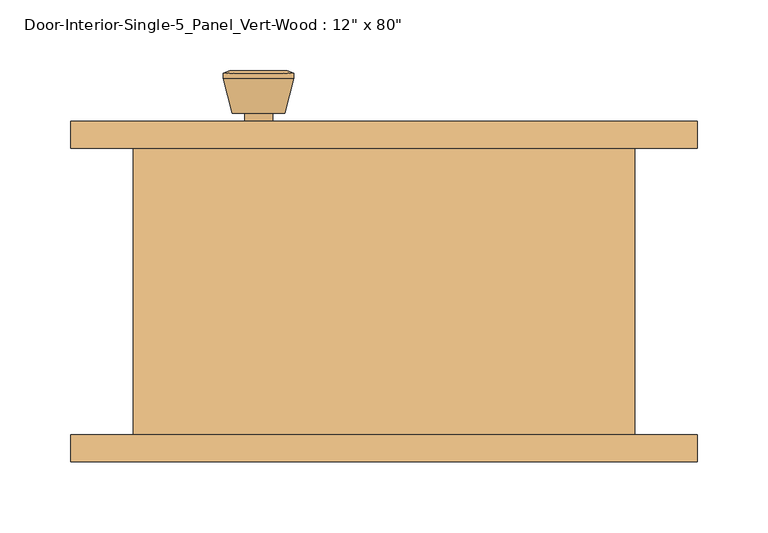
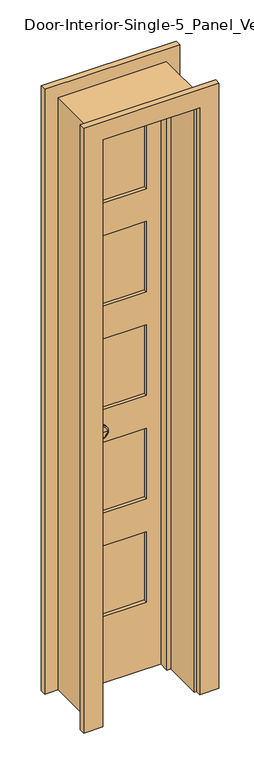
"""IFC4 building model written with IfcOpenShell, lengths in millimetres: door geometry."""

from ifc_helpers import new_model, si_unit, point, frame, frame_2d, origin, place, context, project, spatial, polyline, circle_curve, trimmed, segment, composite_curve, outline, extrude, faceted_brep, source, transform, mapped, element, save
from ifc_brep_helpers import plane_surface, cylinder_surface, revolved_surface, advanced_brep


def door_5a382651(model_context):
    return source(origin(), model_context, "Body", "SolidModel", [
        advanced_brep(
        [(-88.9, 57.5, 914.4), (-78.9, 57.5, 914.4), (-98.9, 57.5, 914.4), (-68.4241324, 8.5, 914.4), (-88.9, 8.5, 914.4), (-109.3758676, 8.5, 914.4), (-63.9, 10.3278681, 914.4), (-113.9, 10.3278681, 914.4), (-63.9, 13.7915463, 914.4), (-113.9, 13.7915463, 914.4), (-70.263764, 38.5, 914.4), (-107.536236, 38.5, 914.4), (-78.9, 38.5, 914.4), (-98.9, 38.5, 914.4)],
        [
            (0, 1),
            (1, 2, circle_curve(frame((-88.9, 57.5, 914.4), z_axis=(0.0, 1.0, 0.0), x_axis=(-1.0, 0.0, 0.0)), 10.0)),
            (2, 0),
            (2, 1, circle_curve(frame((-88.9, 57.5, 914.4), z_axis=(0.0, 1.0, 0.0), x_axis=(-1.0, 0.0, 0.0)), 10.0)),
            (3, 4),
            (4, 5),
            (5, 3, circle_curve(frame((-88.9, 8.5, 914.4), z_axis=(0.0, -1.0, 0.0), x_axis=(-1.0, 0.0, 0.0)), 20.4758676)),
            (3, 5, circle_curve(frame((-88.9, 8.5, 914.4), z_axis=(0.0, -1.0, 0.0), x_axis=(-1.0, 0.0, 0.0)), 20.4758676)),
            (6, 3),
            (5, 7),
            (7, 6, circle_curve(frame((-88.9, 10.3278681, 914.4), z_axis=(0.0, -1.0, 0.0), x_axis=(-1.0, 0.0, 0.0)), 25.0)),
            (6, 7, circle_curve(frame((-88.9, 10.3278681, 914.4), z_axis=(0.0, -1.0, 0.0), x_axis=(-1.0, 0.0, 0.0)), 25.0)),
            (8, 6),
            (7, 9),
            (9, 8, circle_curve(frame((-88.9, 13.7915463, 914.4), z_axis=(0.0, -1.0, 0.0), x_axis=(-1.0, 0.0, 0.0)), 25.0)),
            (8, 9, circle_curve(frame((-88.9, 13.7915463, 914.4), z_axis=(0.0, -1.0, 0.0), x_axis=(-1.0, 0.0, 0.0)), 25.0)),
            (10, 8),
            (9, 11),
            (11, 10, circle_curve(frame((-88.9, 38.5, 914.4), z_axis=(0.0, -1.0, 0.0), x_axis=(-1.0, 0.0, 0.0)), 18.636236)),
            (10, 11, circle_curve(frame((-88.9, 38.5, 914.4), z_axis=(0.0, -1.0, 0.0), x_axis=(-1.0, 0.0, 0.0)), 18.636236)),
            (12, 10),
            (11, 13),
            (13, 12, circle_curve(frame((-88.9, 38.5, 914.4), z_axis=(0.0, -1.0, 0.0), x_axis=(-1.0, 0.0, 0.0)), 10.0)),
            (12, 13, circle_curve(frame((-88.9, 38.5, 914.4), z_axis=(0.0, -1.0, 0.0), x_axis=(-1.0, 0.0, 0.0)), 10.0)),
            (1, 12),
            (13, 2),
        ],
        [
            plane_surface(frame((-88.9, 57.5, 914.4), z_axis=(0.0, 1.0, 0.0), x_axis=(-1.0, 0.0, 0.0))),
            plane_surface(frame((-88.9, 8.5, 914.4), z_axis=(0.0, -1.0, 0.0), x_axis=(-1.0, 0.0, 0.0))),
            revolved_surface(polyline([(-109.3758676, 8.5, 914.4), (-113.9, 10.3278681, 914.4)]), (-88.9, 57.5, 914.4), (0.0, 1.0, 0.0)),
            cylinder_surface(frame((-88.9, 57.5, 914.4), z_axis=(0.0, 1.0, 0.0), x_axis=(-1.0, 0.0, 0.0)), 25.0),
            revolved_surface(polyline([(-113.9, 13.7915463, 914.4), (-107.536236, 38.5, 914.4)]), (-88.9, 57.5, 914.4), (0.0, 1.0, 0.0)),
            plane_surface(frame((-88.9, 38.5, 914.4), z_axis=(0.0, 1.0, 0.0), x_axis=(-1.0, 0.0, 0.0))),
            cylinder_surface(frame((-88.9, 57.5, 914.4), z_axis=(0.0, 1.0, 0.0), x_axis=(-1.0, 0.0, 0.0)), 10.0),
        ],
        [
            (0, [[1, 2, 3]]),
            (0, [[-3, 4, -1]]),
            (1, [[5, 6, 7]]),
            (1, [[-6, -5, 8]]),
            (2, [[9, -7, 10, 11]]),
            (2, [[-10, -8, -9, 12]]),
            (3, [[13, -11, 14, 15]]),
            (3, [[-14, -12, -13, 16]]),
            (4, [[17, -15, 18, 19]]),
            (4, [[-18, -16, -17, 20]]),
            (5, [[21, -19, 22, 23]]),
            (5, [[-22, -20, -21, 24]]),
            (6, [[25, -23, 26, -2]]),
            (6, [[-26, -24, -25, -4]]),
        ],
    ),
        extrude(outline(composite_curve([segment(trimmed(circle_curve(frame_2d((914.4, -88.9)), 30.0), [point((914.4, -118.9))], [point((914.4, -58.9))], False, "CARTESIAN"), True, "CONTINUOUS"), segment(trimmed(circle_curve(frame_2d((914.4, -88.9)), 30.0), [point((914.4, -58.9))], [point((914.4, -118.9))], False, "CARTESIAN"), True, "CONTINUOUS")], self_intersect=False)), frame((0.0, 57.5, 0.0), z_axis=(0.0, 1.0, 0.0), x_axis=(0.0, 0.0, 1.0)), (0.0, 0.0, 1.0), 6.0),
        advanced_brep(
        [(-88.9, 104.425, 914.4), (-98.9, 104.425, 914.4), (-78.9, 104.425, 914.4), (-68.4241324, 153.425, 914.4), (-109.3758676, 153.425, 914.4), (-88.9, 153.425, 914.4), (-63.9, 151.5971319, 914.4), (-113.9, 151.5971319, 914.4), (-63.9, 148.1334537, 914.4), (-113.9, 148.1334537, 914.4), (-70.263764, 123.425, 914.4), (-107.536236, 123.425, 914.4), (-78.9, 123.425, 914.4), (-98.9, 123.425, 914.4)],
        [
            (0, 1),
            (1, 2, circle_curve(frame((-88.9, 104.425, 914.4), z_axis=(0.0, -1.0, 0.0), x_axis=(-1.0, 0.0, 0.0)), 10.0)),
            (2, 0),
            (2, 1, circle_curve(frame((-88.9, 104.425, 914.4), z_axis=(0.0, -1.0, 0.0), x_axis=(-1.0, 0.0, 0.0)), 10.0)),
            (3, 4, circle_curve(frame((-88.9, 153.425, 914.4), z_axis=(0.0, 1.0, 0.0), x_axis=(-1.0, 0.0, 0.0)), 20.4758676)),
            (4, 5),
            (5, 3),
            (4, 3, circle_curve(frame((-88.9, 153.425, 914.4), z_axis=(0.0, 1.0, 0.0), x_axis=(-1.0, 0.0, 0.0)), 20.4758676)),
            (6, 7, circle_curve(frame((-88.9, 151.5971319, 914.4), z_axis=(0.0, 1.0, 0.0), x_axis=(-1.0, 0.0, 0.0)), 25.0)),
            (7, 4),
            (3, 6),
            (7, 6, circle_curve(frame((-88.9, 151.5971319, 914.4), z_axis=(0.0, 1.0, 0.0), x_axis=(-1.0, 0.0, 0.0)), 25.0)),
            (8, 9, circle_curve(frame((-88.9, 148.1334537, 914.4), z_axis=(0.0, 1.0, 0.0), x_axis=(-1.0, 0.0, 0.0)), 25.0)),
            (9, 7),
            (6, 8),
            (9, 8, circle_curve(frame((-88.9, 148.1334537, 914.4), z_axis=(0.0, 1.0, 0.0), x_axis=(-1.0, 0.0, 0.0)), 25.0)),
            (10, 11, circle_curve(frame((-88.9, 123.425, 914.4), z_axis=(0.0, 1.0, 0.0), x_axis=(-1.0, 0.0, 0.0)), 18.636236)),
            (11, 9),
            (8, 10),
            (11, 10, circle_curve(frame((-88.9, 123.425, 914.4), z_axis=(0.0, 1.0, 0.0), x_axis=(-1.0, 0.0, 0.0)), 18.636236)),
            (12, 13, circle_curve(frame((-88.9, 123.425, 914.4), z_axis=(0.0, 1.0, 0.0), x_axis=(-1.0, 0.0, 0.0)), 10.0)),
            (13, 11),
            (10, 12),
            (13, 12, circle_curve(frame((-88.9, 123.425, 914.4), z_axis=(0.0, 1.0, 0.0), x_axis=(-1.0, 0.0, 0.0)), 10.0)),
            (1, 13),
            (12, 2),
        ],
        [
            plane_surface(frame((-88.9, 104.425, 914.4), z_axis=(0.0, -1.0, 0.0), x_axis=(-1.0, 0.0, 0.0))),
            plane_surface(frame((-88.9, 153.425, 914.4), z_axis=(0.0, 1.0, 0.0), x_axis=(-1.0, 0.0, 0.0))),
            revolved_surface(polyline([(-109.3758676, 153.425, 914.4), (-113.9, 151.5971319, 914.4)]), (-88.9, 104.425, 914.4), (0.0, -1.0, 0.0)),
            cylinder_surface(frame((-88.9, 104.425, 914.4), z_axis=(0.0, -1.0, 0.0), x_axis=(-1.0, 0.0, 0.0)), 25.0),
            revolved_surface(polyline([(-113.9, 148.1334537, 914.4), (-107.536236, 123.425, 914.4)]), (-88.9, 104.425, 914.4), (0.0, -1.0, 0.0)),
            plane_surface(frame((-88.9, 123.425, 914.4), z_axis=(0.0, -1.0, 0.0), x_axis=(-1.0, 0.0, 0.0))),
            cylinder_surface(frame((-88.9, 104.425, 914.4), z_axis=(0.0, -1.0, 0.0), x_axis=(-1.0, 0.0, 0.0)), 10.0),
        ],
        [
            (0, [[1, 2, 3]]),
            (0, [[-3, 4, -1]]),
            (1, [[5, 6, 7]]),
            (1, [[8, -7, -6]]),
            (2, [[9, 10, -5, 11]]),
            (2, [[12, -11, -8, -10]]),
            (3, [[13, 14, -9, 15]]),
            (3, [[16, -15, -12, -14]]),
            (4, [[17, 18, -13, 19]]),
            (4, [[20, -19, -16, -18]]),
            (5, [[21, 22, -17, 23]]),
            (5, [[24, -23, -20, -22]]),
            (6, [[-2, 25, -21, 26]]),
            (6, [[-4, -26, -24, -25]]),
        ],
    ),
        extrude(outline(composite_curve([segment(trimmed(circle_curve(frame_2d((914.4, -88.9)), 30.0), [point((914.4, -118.9))], [point((914.4, -58.9))], False, "CARTESIAN"), True, "CONTINUOUS"), segment(trimmed(circle_curve(frame_2d((914.4, -88.9)), 30.0), [point((914.4, -58.9))], [point((914.4, -118.9))], False, "CARTESIAN"), True, "CONTINUOUS")], self_intersect=False)), frame((0.0, 98.425, 0.0), z_axis=(0.0, 1.0, 0.0), x_axis=(0.0, 0.0, 1.0)), (0.0, 0.0, 1.0), 6.0),
        extrude(outline(polyline([(92.075, 75.1416667), (-92.075, 75.1416667), (-92.075, 86.7833333), (92.075, 86.7833333), (92.075, 75.1416667)])), frame((0.0, 0.0, 1668.145), z_axis=(0.0, 0.0, 1.0), x_axis=(1.0, 0.0, 0.0)), (0.0, 0.0, 1.0), 244.7925),
        extrude(outline(polyline([(92.075, 75.1416667), (-92.075, 75.1416667), (-92.075, 86.7833333), (92.075, 86.7833333), (92.075, 75.1416667)])), frame((0.0, 0.0, 1309.0525), z_axis=(0.0, 0.0, 1.0), x_axis=(1.0, 0.0, 0.0)), (0.0, 0.0, 1.0), 244.7925),
        extrude(outline(polyline([(92.075, 75.1416667), (-92.075, 75.1416667), (-92.075, 86.7833333), (92.075, 86.7833333), (92.075, 75.1416667)])), frame((0.0, 0.0, 590.8675), z_axis=(0.0, 0.0, 1.0), x_axis=(1.0, 0.0, 0.0)), (0.0, 0.0, 1.0), 244.7925),
        extrude(outline(polyline([(92.075, 75.1416667), (-92.075, 75.1416667), (-92.075, 86.7833333), (92.075, 86.7833333), (92.075, 75.1416667)])), frame((0.0, 0.0, 231.775), z_axis=(0.0, 0.0, 1.0), x_axis=(1.0, 0.0, 0.0)), (0.0, 0.0, 1.0), 244.7925),
        extrude(outline(polyline([(92.075, 75.1416667), (-92.075, 75.1416667), (-92.075, 86.7833333), (92.075, 86.7833333), (92.075, 75.1416667)])), frame((0.0, 0.0, 949.96), z_axis=(0.0, 0.0, 1.0), x_axis=(1.0, 0.0, 0.0)), (0.0, 0.0, 1.0), 244.7925),
        extrude(outline(polyline([(2032.0, -152.4), (0.0, -152.4), (0.0, 152.4), (2032.0, 152.4), (2032.0, -152.4)]), holes=[polyline([(1912.9375, -92.075), (1912.9375, 92.075), (1668.145, 92.075), (1668.145, -92.075), (1912.9375, -92.075)]), polyline([(476.5675, -92.075), (476.5675, 92.075), (231.775, 92.075), (231.775, -92.075), (476.5675, -92.075)]), polyline([(1194.7525, -92.075), (1194.7525, 92.075), (949.96, 92.075), (949.96, -92.075), (1194.7525, -92.075)]), polyline([(1553.845, -92.075), (1553.845, 92.075), (1309.0525, 92.075), (1309.0525, -92.075), (1553.845, -92.075)]), polyline([(835.66, -92.075), (835.66, 92.075), (590.8675, 92.075), (590.8675, -92.075), (835.66, -92.075)])]), frame((0.0, 63.5, 0.0), z_axis=(0.0, 1.0, 0.0), x_axis=(0.0, 0.0, 1.0)), (0.0, 0.0, 1.0), 34.925),
        faceted_brep([(177.8, 98.425, 0.0), (177.8, -104.775, 0.0), (152.4, -104.775, 0.0), (152.4, 28.575, 0.0), (139.7, 28.575, 0.0), (139.7, 63.5, 0.0), (152.4, 63.5, 0.0), (152.4, 98.425, 0.0), (177.8, 98.425, 2057.4), (177.8, -104.775, 2057.4), (-177.8, -104.775, 2057.4), (-177.8, -104.775, 0.0), (-152.4, -104.775, 0.0), (-152.4, -104.775, 2032.0), (152.4, -104.775, 2032.0), (152.4, 28.575, 2032.0), (-152.4, 28.575, 2032.0), (-152.4, 28.575, 0.0), (-139.7, 28.575, 0.0), (-139.7, 28.575, 2019.3), (139.7, 28.575, 2019.3), (139.7, 63.5, 2019.3), (-139.7, 63.5, 2019.3), (-139.7, 63.5, 0.0), (-152.4, 63.5, 0.0), (-152.4, 63.5, 2032.0), (152.4, 63.5, 2032.0), (152.4, 98.425, 2032.0), (-152.4, 98.425, 2032.0), (-152.4, 98.425, 0.0), (-177.8, 98.425, 0.0), (-177.8, 98.425, 2057.4)], [[[0, 1, 2, 3, 4, 5, 6, 7]], [[1, 0, 8, 9]], [[2, 1, 9, 10, 11, 12, 13, 14]], [[3, 2, 14, 15]], [[4, 3, 15, 16, 17, 18, 19, 20]], [[5, 4, 20, 21]], [[6, 5, 21, 22, 23, 24, 25, 26]], [[7, 6, 26, 27]], [[0, 7, 27, 28, 29, 30, 31, 8]], [[9, 8, 31, 10]], [[15, 14, 13, 16]], [[21, 20, 19, 22]], [[27, 26, 25, 28]], [[30, 29, 24, 23, 18, 17, 12, 11]], [[10, 31, 30, 11]], [[16, 13, 12, 17]], [[22, 19, 18, 23]], [[28, 25, 24, 29]]]),
        extrude(outline(polyline([(0.0, 158.75), (0.0, 222.25), (2101.85, 222.25), (2101.85, -222.25), (0.0, -222.25), (0.0, -158.75), (2038.35, -158.75), (2038.35, 158.75), (0.0, 158.75)])), frame((0.0, -123.825, 0.0), z_axis=(0.0, 1.0, 0.0), x_axis=(0.0, 0.0, 1.0)), (0.0, 0.0, 1.0), 19.05),
        extrude(outline(polyline([(0.0, 158.75), (0.0, 222.25), (2101.85, 222.25), (2101.85, -222.25), (0.0, -222.25), (0.0, -158.75), (2038.35, -158.75), (2038.35, 158.75), (0.0, 158.75)])), frame((0.0, 98.425, 0.0), z_axis=(0.0, 1.0, 0.0), x_axis=(0.0, 0.0, 1.0)), (0.0, 0.0, 1.0), 19.05),
    ])


if __name__ == "__main__":
    model = new_model("IFC4")
    model_context = context("Model", 3, world=origin())
    ifc_project = project(units=[si_unit("LENGTHUNIT", "METRE", prefix="MILLI")], contexts=[model_context])
    site = spatial("IfcSite", under=ifc_project)
    building = spatial("IfcBuilding", under=site)
    placement = place(None, origin())
    door_shape = door_5a382651(model_context)
    element("IfcDoor", 1, ObjectType="Door-Interior-Single-5_Panel_Vert-Wood : 12\" x 80\"", at=placement, inside=building, context=model_context, shape_type="MappedRepresentation", body=[
        mapped(door_shape, transform((0.0, 0.0, 0.0), x_axis=(1.0, 0.0, 0.0), y_axis=(0.0, 1.0, 0.0), z_axis=(0.0, 0.0, 1.0))),
    ])
    save(model, "model.ifc")

# Revit data of these elements
# Type "Door-Interior-Single-5_Panel_Vert-Wood : 12\" x 80\""
#   Type Mark = "8"
#   Assembly Code = "C1020300"
#   Analytic Construction = "Wooden"
#   Top Rail = 0' - 4 11/16"
#   Thickness = 0' - 1 3/8"
#   Thermal Resistance (R) = 2.5876 (h·ft²·°F)/BTU
#   Swing Angle [instance default] = 90.00°
#   Stiles = 0' - 2 3/8"
#   Rough Width = 1' - 2"
#   Rough Height = 6' - 9"
#   Intermediate Rail = 0' - 4 1/2"
#   Height = 6' - 8"
#   Width = 1' - 0"
#   Heat Transfer Coefficient (U) = 0.3865 BTU/(h·ft²·°F)
#   Bottom Rail = 0' - 9 1/8"
#   Trim Material = Cherry
#   Panel Material = Cherry
#   Frame Material = Cherry
#   Door Handle Material = Aluminum
#   Visual Light Transmittance = 0
#   Solar Heat Gain Coefficient = 0
#   Wall Closure = (empty or 0)
#   Function = (empty or 0)
# Element 1 (IfcDoor, "Door-Interior-Single-5_Panel_Vert-Wood : 12\" x 80\"")
#   Materials on its faces: "Cherry", "Aluminum"
# Materials
#   "Cherry": class "Wood", colour RGB 226 177 128, transparency 0, Description = "Prunus Serotina", Cost = 0
#   "Aluminum": class "Metal", colour RGB 247 247 247, transparency 0, Description = "Aluminum 6061", Cost = 0
